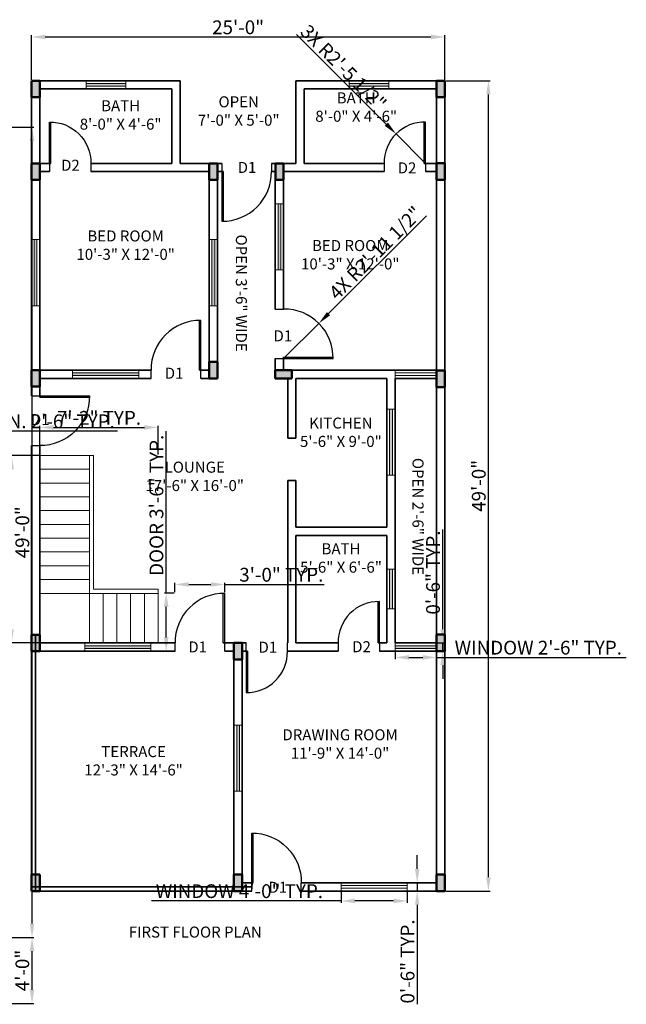
# Model space of a CAD drawing. Units: inches. Extents: x 588 to 1443, y 9704 to 10495.
# Tile 2 of 2: x 1003 to 1443, y 9745 to 10459. Entities that reach past the tile are written whole.
import ezdxf

# ---------------------------------------------------------------- set-up
doc = ezdxf.new("R2010")
doc.units = ezdxf.units.IN
for name, color, linetype, lineweight in [('A-ANNO-DIMS', 2, 'Continuous', 18), ('A-ANNO-TEXT', 7, 'Continuous', 25), ('A-AREA-IDEN', 7, 'Continuous', 18), ('A-COLS', 7, 'Continuous', 50), ('A-DOOR', 3, 'Continuous', 25), ('A-DOOR-IDEN', 3, 'Continuous', 18), ('A-FLOR-STRS', 8, 'Continuous', 18), ('A-GLAZ', 4, 'Continuous', 18), ('A-WALL', 7, 'Continuous', 35)]:
    doc.layers.add(name, color=color, linetype=linetype, lineweight=lineweight)
doc.styles.get("Standard").update_dxf_attribs({"font": 'arial.ttf'})
doc.dimstyles.new('ISO-25', dxfattribs={"dimtxt": 10, "dimasz": 10, "dimexe": 1.25, "dimexo": 0.625, "dimtad": 1, "dimdec": 1, "dimlunit": 3, "dimtxsty": 'Standard', "dimcen": 2.5, "dimadec": 0, "dimazin": 0, "dimtfac": 1, "dimtdec": 1, "dimtmove": 0, "dimatfit": 3, "dimfxl": 1, "dimarcsym": 0})

# ---------------------------------------------------------------- blocks, each defined once
blk = doc.blocks.new('DOOR-SWING-36IN')
for p, q in [((35, 6), (35, 42)), ((36, 6), (36, 42)), ((0, 0), (0, 6)), ((36, 0), (36, 6))]:
    blk.add_line(p, q)
blk.add_arc((35.5, 6.5), 35.5, 89.19307, 180.80693)
blk = doc.blocks.new('DOOR-SWING-30IN')
for p, q in [((0, 30), (0, 36)), ((30, 30), (30, 36)), ((0, 30), (0, 0)), ((1, 30), (1, 0))]:
    blk.add_line(p, q)
blk.add_arc((0.5, 29.5), 29.5, 269.02898, 0.97102)
blk = doc.blocks.new('WIN-48IN')
h = blk.add_hatch(color=256)
h.dxf.hatch_style = 1
h.paths.add_polyline_path([(48, 4), (0, 4), (0, 2), (48, 2)])
for p, q in [((0, 6), (0, 0)), ((0, 4), (48, 4)), ((0, 2), (48, 2)), ((48, 6), (48, 0))]:
    blk.add_line(p, q)
blk = doc.blocks.new('WIN-48IN-OUTLINE')
for p, q in [((0, 6), (0, 0)), ((0, 4), (48, 4)), ((0, 2), (48, 2)), ((48, 6), (48, 0))]:
    blk.add_line(p, q)
blk = doc.blocks.new('WIN-28_8IN')
h = blk.add_hatch(color=256)
h.dxf.hatch_style = 1
h.paths.add_polyline_path([(28.8, 4), (0, 4), (0, 2), (28.8, 2)])
for p, q in [((0, 0), (0, 6)), ((0, 4), (28.8, 4)), ((0, 2), (28.8, 2)), ((28.8, 0), (28.8, 6))]:
    blk.add_line(p, q)
blk = doc.blocks.new('WIN-30IN-OUTLINE')
for p, q in [((0, 0), (0, 6)), ((0, 4), (30, 4)), ((0, 4), (30, 4)), ((0, 2), (30, 2)), ((30, 0), (30, 6))]:
    blk.add_line(p, q)
blk = doc.blocks.new('WIN-30IN')
h = blk.add_hatch(color=256)
h.dxf.hatch_style = 1
h.paths.add_polyline_path([(30, 4), (0, 4), (0, 2), (30, 2)])
for p, q in [((0, 0), (0, 6)), ((0, 4), (30, 4)), ((0, 4), (30, 4)), ((0, 2), (30, 2)), ((30, 0), (30, 6))]:
    blk.add_line(p, q)
blk = doc.blocks.new('COL-6X12IN')
h = blk.add_hatch(color=256)
h.dxf.hatch_style = 1
h.paths.add_polyline_path([(6, 12), (0, 12), (0, 0), (6, 0)])
for p, q in [((0, 12), (6, 12)), ((0, 0), (0, 12)), ((6, 12), (6, 0)), ((6, 0), (0, 0))]:
    blk.add_line(p, q)
blk = doc.blocks.new('STAIR-QUARTER-TURN')
for p, q in [((39, 136), (0, 136)), ((36, 36), (36, 136)), ((39, 39), (39, 136)), ((36, 126), (0, 126)), ((36, 116), (0, 116)), ((36, 106), (0, 106)), ((36, 96), (0, 96)), ((36, 86), (0, 86)), ((36, 76), (0, 76)), ((36, 66), (0, 66)), ((36, 56), (0, 56)), ((36, 46), (0, 46)), ((36, 36), (0, 36)), ((86, 36), (36, 36)), ((36, 36), (36, 0)), ((86, 39), (39, 39)), ((46, 36), (46, 0)), ((56, 36), (56, 0)), ((66, 36), (66, 0)), ((76, 36), (76, 0)), ((86, 39), (86, 0))]:
    blk.add_line(p, q)
blk = doc.blocks.new('*D18')
at = {"layer": 'A-ANNO-DIMS', "color": 0, "lineweight": -2, "transparency": 16777216}
for p, q in [((1109.37, 10042.94), (1109.37, 10160.44)), ((1115.06, 10042.94), (1108.12, 10042.94)), ((1109.37, 10010.8), (1109.37, 10032.94)), ((1115.06, 10000.8), (1108.12, 10000.8))]:
    blk.add_line(p, q, dxfattribs=at)
at = {"layer": 'A-ANNO-DIMS', "color": 0, "transparency": 16777216}
for points in [[(1107.7, 10032.94), (1111.04, 10032.94), (1109.37, 10042.94)], [(1107.7, 10010.8), (1111.04, 10010.8), (1109.37, 10000.8)]]:
    blk.add_solid(points, dxfattribs=at)
at = {"layer": 'Defpoints', "color": 0, "transparency": 16777216}
for p in [(1109.37, 10042.94), (1115.69, 10042.94), (1115.69, 10000.8)]:
    blk.add_point(p, dxfattribs=at)
at = {"layer": 'A-ANNO-DIMS', "color": 0, "transparency": 16777216, "insert": (1103.57, 10106.69), "char_height": 10, "attachment_point": 5, "rotation": 90}
blk.add_mtext('DOOR 3\'-6" TYP.', dxfattribs=at)
blk = doc.blocks.new('*D19')
at = {"layer": 'A-ANNO-DIMS', "color": 0, "lineweight": -2, "transparency": 16777216}
for p, q in [((1115.69, 10043.56), (1115.69, 10050.51)), ((1125.69, 10049.26), (1141.83, 10049.26)), ((1151.83, 10043.56), (1151.83, 10050.51)), ((1151.83, 10049.26), (1224.02, 10049.26))]:
    blk.add_line(p, q, dxfattribs=at)
at = {"layer": 'A-ANNO-DIMS', "color": 0, "transparency": 16777216}
for points in [[(1125.69, 10050.93), (1125.69, 10047.59), (1115.69, 10049.26)], [(1141.83, 10050.93), (1141.83, 10047.59), (1151.83, 10049.26)]]:
    blk.add_solid(points, dxfattribs=at)
at = {"layer": 'Defpoints', "color": 0, "transparency": 16777216}
for p in [(1151.83, 10049.26), (1115.69, 10042.94), (1151.83, 10042.94)]:
    blk.add_point(p, dxfattribs=at)
at = {"layer": 'A-ANNO-DIMS', "color": 0, "transparency": 16777216, "insert": (1192.92, 10054.99), "char_height": 10, "attachment_point": 5}
blk.add_mtext('3\'-0" TYP.', dxfattribs=at)
blk = doc.blocks.new('*D26')
at = {"layer": 'A-ANNO-DIMS', "color": 0, "lineweight": -2, "transparency": 16777216}
for p, q in [((1236.38, 9826.18), (1236.38, 9818.35)), ((1284.38, 9826.18), (1284.38, 9818.35)), ((1236.38, 9819.6), (1098.59, 9819.6)), ((1274.38, 9819.6), (1246.38, 9819.6))]:
    blk.add_line(p, q, dxfattribs=at)
at = {"layer": 'A-ANNO-DIMS', "color": 0, "transparency": 16777216}
for points in [[(1246.38, 9821.27), (1246.38, 9817.94), (1236.38, 9819.6)], [(1274.38, 9821.27), (1274.38, 9817.94), (1284.38, 9819.6)]]:
    blk.add_solid(points, dxfattribs=at)
at = {"layer": 'Defpoints', "color": 0, "transparency": 16777216}
for p in [(1236.38, 9826.8), (1284.38, 9826.8), (1236.38, 9819.6)]:
    blk.add_point(p, dxfattribs=at)
at = {"layer": 'A-ANNO-DIMS', "color": 0, "transparency": 16777216, "insert": (1162.49, 9825.4), "char_height": 10, "attachment_point": 5}
blk.add_mtext('WINDOW 4\'-0" TYP.', dxfattribs=at)
blk = doc.blocks.new('*D27')
at = {"layer": 'A-ANNO-DIMS', "color": 0, "lineweight": -2, "transparency": 16777216}
for p, q in [((1291.58, 9842.8), (1291.58, 9852.8)), ((1285.01, 9832.8), (1292.83, 9832.8)), ((1291.58, 9832.8), (1291.58, 9826.8)), ((1285.01, 9826.8), (1292.83, 9826.8)), ((1291.58, 9816.8), (1291.58, 9744.6))]:
    blk.add_line(p, q, dxfattribs=at)
at = {"layer": 'A-ANNO-DIMS', "color": 0, "transparency": 16777216}
for points in [[(1289.91, 9842.8), (1293.25, 9842.8), (1291.58, 9832.8)], [(1289.91, 9816.8), (1293.25, 9816.8), (1291.58, 9826.8)]]:
    blk.add_solid(points, dxfattribs=at)
at = {"layer": 'Defpoints', "color": 0, "transparency": 16777216}
for p in [(1284.38, 9832.8), (1284.38, 9826.8), (1291.58, 9826.8)]:
    blk.add_point(p, dxfattribs=at)
at = {"layer": 'A-ANNO-DIMS', "color": 0, "transparency": 16777216, "insert": (1285.85, 9775.7), "char_height": 10, "attachment_point": 5, "rotation": 90}
blk.add_mtext('0\'-6" TYP.', dxfattribs=at)
blk = doc.blocks.new('*D28')
at = {"layer": 'A-ANNO-DIMS', "color": 0, "lineweight": -2, "transparency": 16777216}
for p, q in [((936.42, 10164.5), (936.42, 10159.37)), ((946.42, 10160.62), (956.42, 10160.62)), ((966.42, 10164.5), (966.42, 10159.37)), ((966.42, 10160.62), (1073.95, 10160.62))]:
    blk.add_line(p, q, dxfattribs=at)
at = {"layer": 'A-ANNO-DIMS', "color": 0, "transparency": 16777216}
for points in [[(946.42, 10162.29), (946.42, 10158.96), (936.42, 10160.62)], [(956.42, 10162.29), (956.42, 10158.96), (966.42, 10160.62)]]:
    blk.add_solid(points, dxfattribs=at)
at = {"layer": 'Defpoints', "color": 0, "transparency": 16777216}
for p in [(936.42, 10165.12), (966.42, 10165.12), (966.42, 10160.62)]:
    blk.add_point(p, dxfattribs=at)
at = {"layer": 'A-ANNO-DIMS', "color": 0, "transparency": 16777216, "insert": (1025.18, 10166.35), "char_height": 10, "attachment_point": 5}
blk.add_mtext('WIN. 2\'-6" TYP.', dxfattribs=at)
blk = doc.blocks.new('*D30')
at = {"layer": 'A-ANNO-DIMS', "color": 0, "lineweight": -2, "transparency": 16777216}
for p, q in [((1275.57, 10000.18), (1275.57, 9995.05)), ((1285.57, 9996.3), (1295.57, 9996.3)), ((1305.57, 10000.18), (1305.57, 9995.05)), ((1305.57, 9996.3), (1443.36, 9996.3))]:
    blk.add_line(p, q, dxfattribs=at)
at = {"layer": 'A-ANNO-DIMS', "color": 0, "transparency": 16777216}
for points in [[(1285.57, 9997.97), (1285.57, 9994.64), (1275.57, 9996.3)], [(1295.57, 9997.97), (1295.57, 9994.64), (1305.57, 9996.3)]]:
    blk.add_solid(points, dxfattribs=at)
at = {"layer": 'Defpoints', "color": 0, "transparency": 16777216}
for p in [(1275.57, 10000.8), (1305.57, 10000.8), (1305.57, 9996.3)]:
    blk.add_point(p, dxfattribs=at)
at = {"layer": 'A-ANNO-DIMS', "color": 0, "transparency": 16777216, "insert": (1379.46, 10002.1), "char_height": 10, "attachment_point": 5}
blk.add_mtext('WINDOW 2\'-6" TYP.', dxfattribs=at)
blk = doc.blocks.new('*D31')
at = {"layer": 'A-ANNO-DIMS', "color": 0, "lineweight": -2, "transparency": 16777216}
for p, q in [((1310.07, 10016.8), (1310.07, 10089.01)), ((1306.19, 10006.8), (1311.32, 10006.8)), ((1310.07, 10000.8), (1310.07, 10006.8)), ((1306.19, 10000.8), (1311.32, 10000.8)), ((1310.07, 9990.8), (1310.07, 9980.8))]:
    blk.add_line(p, q, dxfattribs=at)
at = {"layer": 'A-ANNO-DIMS', "color": 0, "transparency": 16777216}
for points in [[(1308.4, 10016.8), (1311.73, 10016.8), (1310.07, 10006.8)], [(1308.4, 9990.8), (1311.73, 9990.8), (1310.07, 10000.8)]]:
    blk.add_solid(points, dxfattribs=at)
at = {"layer": 'Defpoints', "color": 0, "transparency": 16777216}
for p in [(1305.57, 10006.8), (1310.07, 10006.8), (1305.57, 10000.8)]:
    blk.add_point(p, dxfattribs=at)
at = {"layer": 'A-ANNO-DIMS', "color": 0, "transparency": 16777216, "insert": (1304.34, 10057.91), "char_height": 10, "attachment_point": 5, "rotation": 90}
blk.add_mtext('0\'-6" TYP.', dxfattribs=at)
blk = doc.blocks.new('*D32')
at = {"layer": 'A-ANNO-DIMS', "color": 0, "lineweight": -2, "transparency": 16777216}
for p, q in [((1016.94, 10142.8), (995.92, 10142.8)), ((997.17, 10016.8), (997.17, 10132.8)), ((1016.94, 10006.8), (995.92, 10006.8))]:
    blk.add_line(p, q, dxfattribs=at)
at = {"layer": 'A-ANNO-DIMS', "color": 0, "transparency": 16777216}
for points in [[(995.5, 10132.8), (998.83, 10132.8), (997.17, 10142.8)], [(995.5, 10016.8), (998.83, 10016.8), (997.17, 10006.8)]]:
    blk.add_solid(points, dxfattribs=at)
at = {"layer": 'Defpoints', "color": 0, "transparency": 16777216}
for p in [(997.17, 10142.8), (1017.57, 10142.8), (1017.57, 10006.8)]:
    blk.add_point(p, dxfattribs=at)
at = {"layer": 'A-ANNO-DIMS', "color": 0, "transparency": 16777216, "insert": (991.37, 10074.8), "char_height": 10, "attachment_point": 5, "rotation": 90}
blk.add_mtext('STAIR 11\'-4" TYP.', dxfattribs=at)
blk = doc.blocks.new('*D33')
at = {"layer": 'A-ANNO-DIMS', "color": 0, "lineweight": -2, "transparency": 16777216}
for p, q in [((1017.57, 10143.43), (1017.57, 10164.45)), ((1027.57, 10163.2), (1093.57, 10163.2)), ((1103.57, 10143.43), (1103.57, 10164.45))]:
    blk.add_line(p, q, dxfattribs=at)
at = {"layer": 'A-ANNO-DIMS', "color": 0, "transparency": 16777216}
for points in [[(1027.57, 10164.87), (1027.57, 10161.54), (1017.57, 10163.2)], [(1093.57, 10164.87), (1093.57, 10161.54), (1103.57, 10163.2)]]:
    blk.add_solid(points, dxfattribs=at)
at = {"layer": 'Defpoints', "color": 0, "transparency": 16777216}
for p in [(1103.57, 10163.2), (1017.57, 10142.8), (1103.57, 10142.8)]:
    blk.add_point(p, dxfattribs=at)
at = {"layer": 'A-ANNO-DIMS', "color": 0, "transparency": 16777216, "insert": (1060.57, 10168.85), "char_height": 10, "attachment_point": 5}
blk.add_mtext('7\'-2" TYP.', dxfattribs=at)
blk = doc.blocks.new('*D34')
at = {"layer": 'A-ANNO-DIMS', "color": 0, "lineweight": -2, "transparency": 16777216}
for p, q in [((967.04, 10381.12), (1013.22, 10381.12)), ((1011.97, 9803.12), (1011.97, 10371.12)), ((967.04, 9793.12), (1013.22, 9793.12))]:
    blk.add_line(p, q, dxfattribs=at)
at = {"layer": 'A-ANNO-DIMS', "color": 0, "transparency": 16777216}
for points in [[(1010.3, 10371.12), (1013.63, 10371.12), (1011.97, 10381.12)], [(1010.3, 9803.12), (1013.63, 9803.12), (1011.97, 9793.12)]]:
    blk.add_solid(points, dxfattribs=at)
at = {"layer": 'Defpoints', "color": 0, "transparency": 16777216}
for p in [(966.42, 10381.12), (1011.97, 10381.12), (966.42, 9793.12)]:
    blk.add_point(p, dxfattribs=at)
at = {"layer": 'A-ANNO-DIMS', "color": 0, "transparency": 16777216, "insert": (1006.24, 10087.12), "char_height": 10, "attachment_point": 5, "rotation": 90}
blk.add_mtext('49\'-0"', dxfattribs=at)
blk = doc.blocks.new('*D35')
at = {"layer": 'A-ANNO-DIMS', "color": 0, "lineweight": -2, "transparency": 16777216}
for p, q in [((967.04, 9793.12), (1013.22, 9793.12)), ((1011.97, 9755.12), (1011.97, 9783.12)), ((973.04, 9745.12), (1013.22, 9745.12))]:
    blk.add_line(p, q, dxfattribs=at)
at = {"layer": 'A-ANNO-DIMS', "color": 0, "transparency": 16777216}
for points in [[(1010.3, 9783.12), (1013.63, 9783.12), (1011.97, 9793.12)], [(1010.3, 9755.12), (1013.63, 9755.12), (1011.97, 9745.12)]]:
    blk.add_solid(points, dxfattribs=at)
at = {"layer": 'Defpoints', "color": 0, "transparency": 16777216}
for p in [(966.42, 9793.12), (1011.97, 9793.12), (972.42, 9745.12)]:
    blk.add_point(p, dxfattribs=at)
at = {"layer": 'A-ANNO-DIMS', "color": 0, "transparency": 16777216, "insert": (1006.24, 9769.12), "char_height": 10, "attachment_point": 5, "rotation": 90}
blk.add_mtext('4\'-0"', dxfattribs=at)
blk = doc.blocks.new('*D38')
at = {"layer": 'A-ANNO-DIMS', "color": 0, "lineweight": -2, "transparency": 16777216}
for p, q in [((1011.57, 10415.43), (1011.57, 10447.75)), ((1021.57, 10446.5), (1301.57, 10446.5)), ((1311.57, 10415.43), (1311.57, 10447.75))]:
    blk.add_line(p, q, dxfattribs=at)
at = {"layer": 'A-ANNO-DIMS', "color": 0, "transparency": 16777216}
for points in [[(1021.57, 10448.17), (1021.57, 10444.84), (1011.57, 10446.5)], [(1301.57, 10448.17), (1301.57, 10444.84), (1311.57, 10446.5)]]:
    blk.add_solid(points, dxfattribs=at)
at = {"layer": 'Defpoints', "color": 0, "transparency": 16777216}
for p in [(1311.57, 10446.5), (1011.57, 10414.8), (1311.57, 10414.8)]:
    blk.add_point(p, dxfattribs=at)
at = {"layer": 'A-ANNO-DIMS', "color": 0, "transparency": 16777216, "insert": (1161.57, 10452.23), "char_height": 10, "attachment_point": 5}
blk.add_mtext('25\'-0"', dxfattribs=at)
blk = doc.blocks.new('*D39')
at = {"layer": 'A-ANNO-DIMS', "color": 0, "lineweight": -2, "transparency": 16777216}
for p, q in [((1312.19, 10414.8), (1344.52, 10414.8)), ((1343.27, 9836.8), (1343.27, 10404.8)), ((1312.19, 9826.8), (1344.52, 9826.8))]:
    blk.add_line(p, q, dxfattribs=at)
at = {"layer": 'A-ANNO-DIMS', "color": 0, "transparency": 16777216}
for points in [[(1341.6, 10404.8), (1344.93, 10404.8), (1343.27, 10414.8)], [(1341.6, 9836.8), (1344.93, 9836.8), (1343.27, 9826.8)]]:
    blk.add_solid(points, dxfattribs=at)
at = {"layer": 'Defpoints', "color": 0, "transparency": 16777216}
for p in [(1311.57, 10414.8), (1343.27, 10414.8), (1311.57, 9826.8)]:
    blk.add_point(p, dxfattribs=at)
at = {"layer": 'A-ANNO-DIMS', "color": 0, "transparency": 16777216, "insert": (1337.54, 10120.8), "char_height": 10, "attachment_point": 5, "rotation": 90}
blk.add_mtext('49\'-0"', dxfattribs=at)
blk = doc.blocks.new('*D42')
at = {"layer": 'A-ANNO-DIMS', "color": 0, "lineweight": -2, "transparency": 16777216}
for p, q in [((1298.21, 10316.73), (1227.24, 10245.76)), ((1195.07, 10213.59), (1220.17, 10238.69))]:
    blk.add_line(p, q, dxfattribs=at)
at = {"layer": 'A-ANNO-DIMS', "color": 0, "transparency": 16777216}
blk.add_solid([(1226.06, 10246.94), (1228.42, 10244.59), (1220.17, 10238.69)], dxfattribs=at)
at = {"layer": 'Defpoints', "color": 0, "transparency": 16777216}
for p in [(1220.17, 10238.69), (1195.07, 10213.59)]:
    blk.add_point(p, dxfattribs=at)
at = {"layer": 'A-ANNO-DIMS', "color": 0, "transparency": 16777216, "insert": (1262.16, 10288.88), "char_height": 10, "attachment_point": 5, "rotation": 44.99929}
blk.add_mtext('4X R2\'-11 1/2"', dxfattribs=at)
blk = doc.blocks.new('*D43')
at = {"layer": 'A-ANNO-DIMS', "color": 0, "lineweight": -2, "transparency": 16777216}
for p, q in [((1203.95, 10448.42), (1269.14, 10383.24)), ((1297.07, 10355.3), (1276.21, 10376.17))]:
    blk.add_line(p, q, dxfattribs=at)
at = {"layer": 'A-ANNO-DIMS', "color": 0, "transparency": 16777216}
blk.add_solid([(1270.32, 10384.42), (1267.96, 10382.06), (1276.21, 10376.17)], dxfattribs=at)
at = {"layer": 'Defpoints', "color": 0, "transparency": 16777216}
for p in [(1276.21, 10376.17), (1297.07, 10355.3)]:
    blk.add_point(p, dxfattribs=at)
at = {"layer": 'A-ANNO-DIMS', "color": 0, "transparency": 16777216, "insert": (1237.11, 10423.47), "char_height": 10, "attachment_point": 5, "rotation": 315.00036}
blk.add_mtext('3X R2\'-5 1/2"', dxfattribs=at)

msp = doc.modelspace()

# ---------------------------------------------------------------- linework, layer by layer
at = {"layer": 'A-WALL'}
for p, q in [((1011.57, 10186.05), (1011.57, 10414.8)), ((1119.57, 10414.8), (1011.57, 10414.8)), ((1119.57, 10354.8), (1119.57, 10414.8)), ((1203.57, 10354.8), (1203.57, 10414.8)), ((1305.57, 10414.8), (1203.57, 10414.8)), ((1311.57, 9827.01), (1311.57, 10414.8)), ((1017.57, 10354.8), (1017.57, 10408.8)), ((1113.57, 10408.8), (1017.57, 10408.8)), ((1113.57, 10354.8), (1113.57, 10408.8)), ((1209.57, 10354.8), (1209.57, 10408.8)), ((1305.57, 10408.8), (1209.57, 10408.8)), ((1305.57, 10354.8), (1305.57, 10408.8)), ((1025.64, 10354.8), (1017.57, 10354.8)), ((1113.57, 10354.8), (1054.64, 10354.8)), ((1149.7, 10354.8), (1119.57, 10354.8)), ((1203.57, 10354.8), (1185.7, 10354.8)), ((1267.57, 10354.8), (1209.57, 10354.8)), ((1305.57, 10354.8), (1296.57, 10354.8)), ((1017.57, 10204.8), (1017.57, 10348.8)), ((1024.64, 10348.8), (1017.57, 10348.8)), ((1113.57, 10348.8), (1054.64, 10348.8)), ((1140.57, 10348.8), (1113.57, 10348.8)), ((1140.57, 10204.8), (1140.57, 10348.8)), ((1146.57, 10198.8), (1146.57, 10348.8)), ((1150.7, 10348.8), (1146.57, 10348.8)), ((1188.57, 10348.8), (1185.7, 10348.8)), ((1188.57, 10249.09), (1188.57, 10348.8)), ((1194.57, 10249.09), (1194.57, 10348.8)), ((1209.57, 10348.8), (1194.57, 10348.8)), ((1267.57, 10348.8), (1209.57, 10348.8)), ((1305.57, 10348.8), (1297.57, 10348.8)), ((1305.57, 10204.8), (1305.57, 10348.8)), ((1188.57, 10198.8), (1188.57, 10213.09)), ((1194.57, 10204.8), (1194.57, 10214.09)), ((1098.42, 10204.8), (1017.57, 10204.8)), ((1140.57, 10204.8), (1133.42, 10204.8)), ((1305.57, 10204.8), (1194.57, 10204.8)), ((1017.57, 10185.05), (1017.57, 10198.8)), ((1098.42, 10198.8), (1017.57, 10198.8)), ((1146.57, 10198.8), (1134.42, 10198.8)), ((1197.57, 10198.8), (1188.57, 10198.8)), ((1197.57, 10155.28), (1197.57, 10198.8)), ((1203.57, 10155.28), (1203.57, 10198.8)), ((1269.57, 10198.8), (1203.57, 10198.8)), ((1269.57, 10090.8), (1269.57, 10198.8)), ((1275.57, 10006.8), (1275.57, 10198.8)), ((1305.57, 10198.8), (1275.57, 10198.8)), ((1305.57, 10006.8), (1305.57, 10198.8)), ((1197.57, 10155.28), (1203.57, 10155.28)), ((1011.57, 9826.8), (1011.57, 10150.05)), ((1017.57, 10006.8), (1017.57, 10150.05)), ((1197.57, 10006.8), (1197.57, 10124.65)), ((1197.57, 10124.65), (1203.57, 10124.65)), ((1203.57, 10090.8), (1203.57, 10124.65)), ((1269.57, 10090.8), (1203.57, 10090.8)), ((1203.57, 10006.8), (1203.57, 10084.8)), ((1269.57, 10084.8), (1203.57, 10084.8)), ((1269.57, 10006.8), (1269.57, 10084.8)), ((1014.57, 9826.8), (1014.57, 10012.8)), ((1115.83, 10006.8), (1017.57, 10006.8)), ((1158.57, 10006.8), (1150.83, 10006.8)), ((1158.57, 10006.8), (1167.37, 10006.8)), ((1197.37, 10006.8), (1197.57, 10006.8)), ((1234.12, 10006.8), (1203.57, 10006.8)), ((1269.57, 10006.8), (1263.12, 10006.8)), ((1305.57, 10006.8), (1275.57, 10006.8)), ((1115.83, 10000.8), (1011.57, 10000.8)), ((1158.57, 10000.8), (1151.83, 10000.8)), ((1158.57, 9826.8), (1158.57, 10000.8)), ((1164.57, 9832.8), (1164.57, 10000.8)), ((1164.57, 10000.8), (1168.37, 10000.8)), ((1197.37, 10000.8), (1197.57, 10000.8)), ((1234.12, 10000.8), (1197.57, 10000.8)), ((1305.57, 10000.8), (1264.12, 10000.8)), ((1305.57, 9832.8), (1305.57, 10000.8)), ((1172.43, 9832.8), (1164.57, 9832.8)), ((1305.57, 9832.8), (1207.43, 9832.8)), ((1171.43, 9829.8), (1011.57, 9829.8)), ((1171.43, 9826.8), (1011.57, 9826.8)), ((1305.57, 9826.8), (1207.43, 9826.8))]:
    msp.add_line(p, q, dxfattribs=at)

# ---------------------------------------------------------------- block references
at = {"layer": 'A-COLS'}
for p in [(1011.57, 10402.8), (1305.57, 10402.8), (1011.57, 10342.8), (1140.49, 10342.8), (1188.63, 10342.8), (1305.57, 10342.88), (1140.57, 10198.8), (1011.57, 10192.8), (1305.57, 10192.47), (1011.57, 10000.8), (1305.57, 10000.84), (1158.57, 9994.8), (1011.57, 9826.8), (1158.57, 9826.74), (1305.57, 9826.8)]:
    msp.add_blockref('COL-6X12IN', p, dxfattribs=at)
at = {"layer": 'A-COLS', "rotation": 90.00000000000885}
msp.add_blockref('COL-6X12IN', (1200.57, 10198.8), dxfattribs=at)
at = {"layer": 'A-DOOR', "extrusion": (0, 0, -1), "zscale": -1}
for name, p, rotation in [('DOOR-SWING-30IN', (-1024.64, 10384.81), 180), ('DOOR-SWING-36IN', (-1011.57, 10150.04), 90.0000000000085)]:
    msp.add_blockref(name, p, dxfattribs=dict(at, rotation=rotation))
at = {"layer": 'A-DOOR'}
for name, p, rotation in [('DOOR-SWING-30IN', (1297.57, 10384.81), 180), ('DOOR-SWING-36IN', (1185.7, 10354.8), 180), ('DOOR-SWING-36IN', (1188.57, 10249.09), 270.0000000000084), ('DOOR-SWING-30IN', (1264.12, 10036.81), 180)]:
    msp.add_blockref(name, p, dxfattribs=dict(at, rotation=rotation))
for name, p in [('DOOR-SWING-36IN', (1098.42, 10198.8)), ('DOOR-SWING-36IN', (1115.82, 10000.8)), ('DOOR-SWING-30IN', (1167.37, 9970.8))]:
    msp.add_blockref(name, p, dxfattribs=at)
at = {"layer": 'A-DOOR', "extrusion": (0, 0, -1), "zscale": -1}
msp.add_blockref('DOOR-SWING-36IN', (-1207.43, 9826.8), dxfattribs=at)
at = {"layer": 'A-FLOR-STRS'}
msp.add_blockref('STAIR-QUARTER-TURN', (1017.57, 10006.8), dxfattribs=at)
at = {"layer": 'A-GLAZ'}
for name, p in [('WIN-28_8IN', (1051.17, 10408.8)), ('WIN-28_8IN', (1242.21, 10408.8)), ('WIN-48IN', (1041.41, 10198.8)), ('WIN-30IN-OUTLINE', (1275.57, 10198.8)), ('WIN-48IN', (1050.28, 10000.8)), ('WIN-30IN', (1275.57, 10000.8))]:
    msp.add_blockref(name, p, dxfattribs=at)
at = {"layer": 'A-GLAZ', "extrusion": (0, 0, -1), "zscale": -1}
for name, p, rotation in [('WIN-48IN', (-1188.57, 10277.53), 89.99999999999602), ('WIN-48IN', (-1011.57, 10251.45), 89.99999999999577), ('WIN-48IN', (-1140.57, 10251.45), 89.99999999999602), ('WIN-48IN', (-1269.57, 10128.46), 89.99999999999648), ('WIN-28_8IN', (-1269.57, 10031.45), 90.00000000002223), ('WIN-48IN', (-1158.57, 9899.15), 89.99999999999648)]:
    msp.add_blockref(name, p, dxfattribs=dict(at, rotation=rotation))
at = {"layer": 'A-GLAZ', "rotation": 180}
msp.add_blockref('WIN-48IN-OUTLINE', (1284.38, 9832.8), dxfattribs=at)

# ---------------------------------------------------------------- texts
at = {"layer": 'A-ANNO-TEXT', "insert": (1082.21, 9801.01), "char_height": 8, "attachment_point": 1}
msp.add_mtext_dynamic_manual_height_columns('{\\fArial|b1|i0|c0|p34;FIRST FLOOR PLAN}', width=233.0578, gutter_width=12.5, heights=[0], dxfattribs=at)
at = {"layer": 'A-AREA-IDEN', "char_height": 8, "attachment_point": 1}
for s, width, insert in [('\\pxqc;OPEN\\P7\'-0" X 5\'-0"', 96.8159, (1113.57, 10403.45)), ('\\pxqc;BATH\\P8\'-0" X 4\'-6"', 87.4066, (1203.57, 10406.31)), ('\\pxqc;BATH\\P8\'-0" X 4\'-6"', 87.4066, (1032.59, 10400.59)), ('\\pxqc;BED ROOM\\P10\'-3" X 12\'-0"', 96.8159, (1031.51, 10306.13)), ('\\pxqc;BED ROOM\\P10\'-3" X 12\'-0"', 96.8159, (1194.57, 10299.18)), ('\\pxqc;KITCHEN\\P5\'-6" X 9\'-0"', 96.8159, (1187.75, 10170.37)), ('\\pxqc;LOUNGE\\P17\'-6" X 16\'-0"', 96.8159, (1081.66, 10138.36)), ('\\pxqc;BATH\\P5\'-6" X 6\'-6"', 96.8159, (1187.86, 10079.12)), ('\\pxqc;DRAWING ROOM\\P11\'-9" X 14\'-0"', 96.8159, (1187.15, 9944.16)), ('\\pxqc;TERRACE\\P12\'-3" X 14\'-6"', 96.8159, (1037.27, 9931.98))]:
    msp.add_mtext_dynamic_manual_height_columns(s, width=width, gutter_width=12.5, heights=[0], dxfattribs=dict(at, insert=insert))
at = {"layer": 'A-AREA-IDEN', "char_height": 8, "attachment_point": 1, "rotation": 270}
for s, insert in [('OPEN 3\'-6" WIDE', (1167.92, 10303.17)), ('OPEN 2\'-6" WIDE', (1296.15, 10141.09))]:
    msp.add_mtext_dynamic_manual_height_columns(s, width=203.6948, gutter_width=12.5, heights=[0], dxfattribs=dict(at, insert=insert))
at = {"layer": 'A-DOOR-IDEN', "char_height": 8, "attachment_point": 1}
for s, insert in [('D2', (1033.05, 10357.43)), ('D1', (1161.24, 10355.84)), ('D2', (1277.39, 10355.51)), ('D1', (1187.26, 10233.64)), ('D1', (1108.31, 10206.55)), ('D1', (1011.14, 10172.91)), ('D1', (1125.42, 10007.92)), ('D1', (1176.36, 10007.73)), ('D2', (1244.38, 10008.07)), ('D1', (1183.57, 9833.5))]:
    msp.add_mtext_dynamic_manual_height_columns(s, width=15.8534, gutter_width=12.5, heights=[9.35], dxfattribs=dict(at, insert=insert))

# ---------------------------------------------------------------- dimensions: what is measured, and where the dimension line sits
at = {"layer": 'A-ANNO-DIMS'}
dim = msp.add_linear_dim(base=(1311.57, 10446.5), p1=(1011.57, 10414.8), p2=(1311.57, 10414.8), dimstyle='ISO-25', override={"dimdec": 1, "dimlfac": 1, "dimrnd": 0, "dimzin": 1, "dimdsep": 46, "dimlunit": 4, "dimfrac": 2}, dxfattribs=at)
dim.commit()
dim.dimension.update_dxf_attribs({"geometry": '*D38', "text_midpoint": (1161.57, 10452.23)})
for center, mpoint, text, picture, middle in [((1297.07, 10355.3), (1276.21, 10376.17), '3X <>', '*D43', (1237.11, 10423.47)), ((1195.07, 10213.59), (1220.17, 10238.69), '4X <>', '*D42', (1262.16, 10288.88))]:
    dim = msp.add_radius_dim(center=center, mpoint=mpoint, text=text, dimstyle='ISO-25', override={"dimdec": 1, "dimlfac": 1, "dimrnd": 0, "dimzin": 1, "dimdsep": 46, "dimlunit": 4, "dimfrac": 2}, dxfattribs=at)
    dim.commit()
    dim.dimension.update_dxf_attribs({"geometry": picture, "text_midpoint": middle})
for base, p1, p2, picture, middle in [((1343.27, 10414.8), (1311.57, 9826.8), (1311.57, 10414.8), '*D39', (1337.54, 10120.8)), ((1011.97, 10381.12), (966.42, 9793.12), (966.42, 10381.12), '*D34', (1006.24, 10087.12)), ((1011.97, 9793.12), (972.42, 9745.12), (966.42, 9793.12), '*D35', (1006.24, 9769.12))]:
    dim = msp.add_linear_dim(base=base, p1=p1, p2=p2, angle=90, dimstyle='ISO-25', override={"dimdec": 1, "dimlfac": 1, "dimrnd": 0, "dimzin": 1, "dimdsep": 46, "dimlunit": 4, "dimfrac": 2}, dxfattribs=at)
    dim.commit()
    dim.dimension.update_dxf_attribs({"geometry": picture, "text_midpoint": middle})
for base, p1, p2, text, picture, middle in [((966.42, 10160.62), (936.42, 10165.12), (966.42, 10165.12), 'WIN. <> TYP.', '*D28', (1025.18, 10166.35)), ((1103.57, 10163.2), (1017.57, 10142.8), (1103.57, 10142.8), '<> TYP.', '*D33', (1060.57, 10168.85)), ((1151.83, 10049.26), (1115.69, 10042.94), (1151.83, 10042.94), '<> TYP.', '*D19', (1192.92, 10054.99)), ((1305.57, 9996.3), (1275.57, 10000.8), (1305.57, 10000.8), 'WINDOW <> TYP.', '*D30', (1379.46, 10002.1))]:
    dim = msp.add_linear_dim(base=base, p1=p1, p2=p2, text=text, dimstyle='ISO-25', override={"dimdec": 1, "dimlfac": 1, "dimrnd": 0, "dimzin": 1, "dimdsep": 46, "dimlunit": 4, "dimfrac": 2}, dxfattribs=at)
    dim.commit()
    dim.dimension.update_dxf_attribs({"geometry": picture, "text_midpoint": middle})
for base, p1, p2, angle, text, picture, middle in [((1109.37, 10042.94), (1115.69, 10000.8), (1115.69, 10042.94), 90, 'DOOR <> TYP.', '*D18', (1103.57, 10106.69)), ((997.17, 10142.8), (1017.57, 10006.8), (1017.57, 10142.8), 90, 'STAIR <> TYP.', '*D32', (991.37, 10074.8)), ((1310.07, 10006.8), (1305.57, 10000.8), (1305.57, 10006.8), 90, '<> TYP.', '*D31', (1304.34, 10057.91)), ((1291.58, 9826.8), (1284.38, 9832.8), (1284.38, 9826.8), 270, '<> TYP.', '*D27', (1285.85, 9775.7)), ((1236.38, 9819.6), (1284.38, 9826.8), (1236.38, 9826.8), 180, 'WINDOW <> TYP.', '*D26', (1162.49, 9825.4))]:
    dim = msp.add_linear_dim(base=base, p1=p1, p2=p2, angle=angle, text=text, dimstyle='ISO-25', override={"dimdec": 1, "dimlfac": 1, "dimrnd": 0, "dimzin": 1, "dimdsep": 46, "dimlunit": 4, "dimfrac": 2}, dxfattribs=at)
    dim.commit()
    dim.dimension.update_dxf_attribs({"geometry": picture, "text_midpoint": middle})

doc.saveas('drawing.dxf')
